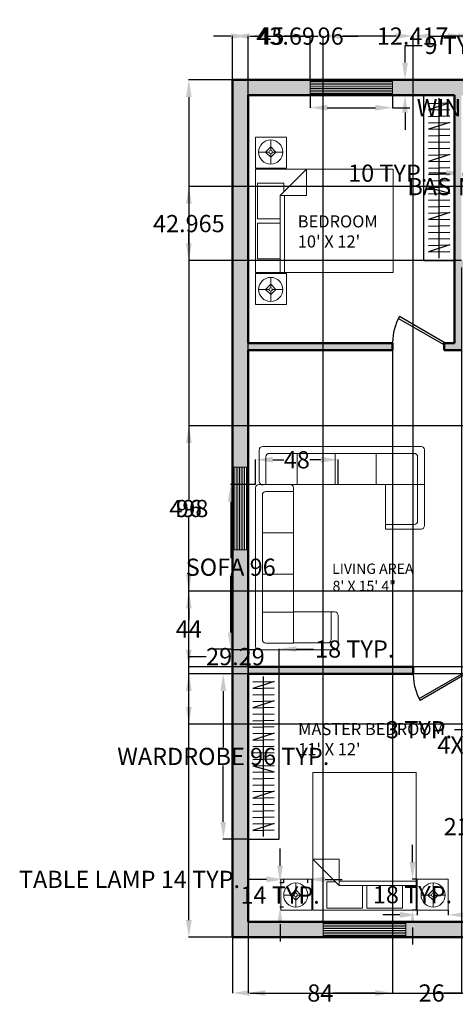
# Model space of a CAD drawing. Units: inches. Extents: x 133 to 758, y -29 to 543.
# Tile 1 of 7: x 133 to 386, y -29 to 543. Entities that reach past the tile are written whole.
import ezdxf

# ---------------------------------------------------------------- set-up
doc = ezdxf.new("R2010")
doc.units = ezdxf.units.IN
doc.header["$MEASUREMENT"] = 0
for name, color, linetype, lineweight in [('A-ANNO-DIMS', 2, 'Continuous', 18), ('A-AREA-IDEN', 7, 'Continuous', 25), ('A-FLOR-CASE', 32, 'Continuous', 25), ('A-FURN', 8, 'Continuous', 18), ('A-WALL', 7, 'Continuous', 50), ('DOOR', 40, 'Continuous', 25), ('WINDOW', 151, 'Continuous', 18)]:
    doc.layers.add(name, color=color, linetype=linetype, lineweight=lineweight)
doc.layers.add('A-WALL-PATT', color=251, linetype='Continuous', lineweight=13, true_color=0x636466)
doc.styles.get("Standard").update_dxf_attribs({"font": 'arial.ttf'})
doc.dimstyles.get("Standard").update_dxf_attribs({"dimtxt": 10, "dimasz": 10, "dimexe": 0.18, "dimexo": 0.0625, "dimgap": 0.09, "dimtad": 0, "dimtih": 1, "dimtoh": 1, "dimdec": 0, "dimzin": 0, "dimdsep": 46, "dimlunit": 4, "dimtxsty": 'Standard', "dimcen": 0.09, "dimadec": 0, "dimazin": 0, "dimtfac": 1, "dimtdec": 0, "dimtofl": 0, "dimtmove": 0, "dimatfit": 3, "dimfxl": 1, "dimtolj": 1, "dimtzin": 0, "dimarcsym": 0})

# ---------------------------------------------------------------- blocks, each defined once
blk = doc.blocks.new('*U14')
for p, q in [((0, 0), (0, -6)), ((-40, 0), (-40, -6))]:
    blk.add_line(p, q)
blk.add_lwpolyline([(0, 0), (-34.64, 20), (-35.52, 18.48), (-0.88, -1.52)], close=True)
blk.add_arc((0, 0), 40, 150, 180)
blk = doc.blocks.new('*U12')
for p, q in [((-40, 0), (-40, 6)), ((0, 0), (0, 6))]:
    blk.add_line(p, q)
blk.add_lwpolyline([(0, 0), (-34.64, -20), (-35.52, -18.48), (-0.88, 1.52)], close=True)
blk.add_arc((0, 0), 40, 180, 210)
blk = doc.blocks.new('SOFA')
for p, q in [((-1, 0), (1, 0)), ((1, 0), (17, 0)), ((-3, -2), (-3, -94)), ((19, -4), (3, -4)), ((19, -2), (19, -4)), ((43, -74), (41, -74)), ((41, -74), (41, -90)), ((45, -92), (45, -76)), ((-1, -96), (43, -96)), ((45, -92), (45, -94))]:
    blk.add_line(p, q)
blk.add_lwpolyline([(3, -4), (19.13, -4), (19.13, -28), (1, -28), (1, -6, -0.414214)], format="xyb", close=True)
for points in [[(39, -92), (19.13, -92), (19.13, -92.1), (3, -92.1, -0.414214), (1, -90.1), (1, -6)], [(1, -74.06), (19.13, -74.06), (19.13, -92), (39, -92, 0.414214), (41, -90), (41, -74), (19.13, -74), (19.13, -52), (1, -52), (1, -76)]]:
    blk.add_lwpolyline(points, format="xyb")
blk.add_lwpolyline([(1, -28), (19.13, -28), (19.13, -52), (1, -52)], close=True)
for centre, start, end in [((-1, -2), 90, 180), ((17, -2), 0, 90), ((43, -76), 0, 90), ((-1, -94), 180, 270), ((43, -94), 270, 0)]:
    blk.add_arc(centre, 2, start, end)
blk = doc.blocks.new('Bed - Queen')
for p, q in [((0, -80.00003), (0, 0)), ((0, 0), (59.99999, 0)), ((59.99999, 0), (59.99999, -80.00003)), ((7.99999, -1.2), (28.79998, -1.2)), ((7.99999, -14.4), (7.99999, -1.2)), ((28.79998, -1.2), (28.79998, -14.4)), ((31.19999, -1.2), (51.99999, -1.2)), ((31.19999, -14.4), (31.19999, -1.2)), ((51.99999, -1.2), (51.99999, -16.4)), ((0, -14.4), (44.8, -14.4)), ((44.8, -16.8), (0, -16.8)), ((59.99999, -29.6), (44.8, -14.4)), ((44.8, -14.4), (44.8, -29.6)), ((51.99999, -16.4), (46.79936, -16.4)), ((44.8, -29.6), (59.99999, -29.6)), ((59.99999, -80.00003), (0, -80.00003))]:
    blk.add_line(p, q)
blk = doc.blocks.new('Lamp - Table')
for p, q in [((0, 7), (0, 1)), ((-1, 0), (-7, 0)), ((0, 3), (-3, 0)), ((-3, 0), (0, -3)), ((3, 0), (0, 3)), ((0, -3), (3, 0)), ((1, 0), (7, 0)), ((0, -1), (0, -7))]:
    blk.add_line(p, q)
for radius in [7, 1]:
    blk.add_circle((0, 0), radius)
blk = doc.blocks.new('WIN-48IN')
for p, q in [((0, 8), (48, 8)), ((0, 7), (48, 7)), ((0, 6), (48, 6)), ((0, 5), (48, 5)), ((0, 4), (48, 4)), ((0, 3), (48, 3)), ((0, 2), (48, 2)), ((0, 1), (48, 1)), ((0, 0), (48, 0))]:
    blk.add_line(p, q)
blk.add_lwpolyline([(48, 9), (48, 0), (0, 0), (0, 9)], close=True)
blk = doc.blocks.new('WARDROBE-96X18IN')
for p, q in [((18, 96), (0, 96)), ((0, 96), (0, 0)), ((2.8, 91.24), (15.16, 91.53)), ((15.16, 91.53), (2.8, 87.49)), ((9, 1.47), (9, 94.4)), ((18, 0), (18, 96)), ((2.8, 87.49), (15.16, 87.78)), ((2.8, 83.75), (15.16, 84.04)), ((2.8, 80), (15.16, 80.29)), ((15.16, 80.29), (2.8, 76.25)), ((2.8, 76.25), (15.16, 76.54)), ((2.8, 72.51), (15.16, 72.8)), ((2.8, 68.76), (15.16, 69.05)), ((2.8, 65.01), (15.16, 65.3)), ((2.8, 61.27), (15.16, 61.56)), ((15.16, 61.56), (2.8, 57.52)), ((2.8, 57.52), (15.16, 57.81)), ((2.8, 53.77), (15.16, 54.06)), ((2.8, 50.03), (15.16, 50.32)), ((2.8, 46.28), (15.16, 46.57)), ((2.8, 42.53), (15.16, 42.82)), ((2.8, 42.53), (15.16, 39.08)), ((2.8, 38.79), (15.16, 39.08)), ((2.8, 35.04), (15.16, 35.33)), ((2.8, 31.29), (15.16, 31.58)), ((2.8, 27.55), (15.16, 27.84)), ((15.16, 27.84), (2.8, 23.8)), ((2.8, 23.8), (15.16, 24.09)), ((2.8, 20.06), (15.16, 20.35)), ((2.8, 16.31), (15.16, 16.6)), ((2.8, 12.56), (15.16, 12.85)), ((2.8, 8.82), (15.16, 9.11)), ((15.16, 9.11), (2.8, 5.07)), ((0, 0), (18, 0)), ((2.8, 5.07), (15.16, 5.36))]:
    blk.add_line(p, q)
blk = doc.blocks.new('NIGHTSTAND-18IN')
blk.add_lwpolyline([(18, 18), (18, 0), (0, 0), (0, 18)], close=True)
blk = doc.blocks.new('*D38')
at = {"layer": 'A-ANNO-DIMS', "color": 0, "lineweight": -2, "transparency": 16777216}
for p, q in [((276.46, 43.94), (266.46, 43.94)), ((286.46, 41.9), (286.46, 44.12)), ((300.46, 41.9), (300.46, 44.12)), ((310.46, 43.94), (320.46, 43.94))]:
    blk.add_line(p, q, dxfattribs=at)
at = {"layer": 'A-ANNO-DIMS', "color": 0, "transparency": 16777216}
for points in [[(276.46, 45.6), (276.46, 42.27), (286.46, 43.94)], [(310.46, 45.6), (310.46, 42.27), (300.46, 43.94)]]:
    blk.add_solid(points, dxfattribs=at)
at = {"layer": 'Defpoints', "color": 0, "transparency": 16777216}
for p in [(286.46, 43.94), (286.46, 41.84), (300.46, 41.84)]:
    blk.add_point(p, dxfattribs=at)
at = {"layer": 'A-ANNO-DIMS', "color": 0, "transparency": 16777216, "insert": (196.87, 43.94), "char_height": 10, "attachment_point": 5}
blk.add_mtext('\\A1;TABLE LAMP 14 TYP.', dxfattribs=at)
blk = doc.blocks.new('*D39')
at = {"layer": 'A-ANNO-DIMS', "color": 0, "lineweight": -2, "transparency": 16777216}
for p, q in [((284.36, 51.84), (284.36, 61.84)), ((286.4, 41.84), (284.18, 41.84)), ((286.4, 27.84), (284.18, 27.84)), ((284.36, 17.84), (284.36, 7.84))]:
    blk.add_line(p, q, dxfattribs=at)
at = {"layer": 'A-ANNO-DIMS', "color": 0, "transparency": 16777216}
for points in [[(282.69, 51.84), (286.02, 51.84), (284.36, 41.84)], [(282.69, 17.84), (286.02, 17.84), (284.36, 27.84)]]:
    blk.add_solid(points, dxfattribs=at)
at = {"layer": 'Defpoints', "color": 0, "transparency": 16777216}
for p in [(286.46, 41.84), (284.36, 27.84), (286.46, 27.84)]:
    blk.add_point(p, dxfattribs=at)
at = {"layer": 'A-ANNO-DIMS', "color": 0, "transparency": 16777216, "insert": (284.36, 34.84), "char_height": 10, "attachment_point": 5}
blk.add_mtext('\\A1;14 TYP.', dxfattribs=at)
blk = doc.blocks.new('*D40')
at = {"layer": 'A-ANNO-DIMS', "color": 0, "lineweight": -2, "transparency": 16777216}
for p, q in [((353.97, 23.32), (343.97, 23.32)), ((363.97, 25.96), (363.97, 23.14)), ((381.97, 25.96), (381.97, 23.14)), ((391.97, 23.32), (401.97, 23.32))]:
    blk.add_line(p, q, dxfattribs=at)
at = {"layer": 'A-ANNO-DIMS', "color": 0, "transparency": 16777216}
for points in [[(353.97, 24.99), (353.97, 21.65), (363.97, 23.32)], [(391.97, 24.99), (391.97, 21.65), (381.97, 23.32)]]:
    blk.add_solid(points, dxfattribs=at)
at = {"layer": 'Defpoints', "color": 0, "transparency": 16777216}
for p in [(363.97, 26.02), (381.97, 26.02), (381.97, 23.32)]:
    blk.add_point(p, dxfattribs=at)
at = {"layer": 'A-ANNO-DIMS', "color": 0, "transparency": 16777216, "insert": (473.5, 23.32), "char_height": 10, "attachment_point": 5}
blk.add_mtext('\\A1;NIGHTSTAND 18 TYP.', dxfattribs=at)
blk = doc.blocks.new('*D41')
at = {"layer": 'A-ANNO-DIMS', "color": 0, "lineweight": -2, "transparency": 16777216}
for p, q in [((361.27, 54.02), (361.27, 64.02)), ((363.9, 44.02), (361.09, 44.02)), ((363.9, 26.02), (361.09, 26.02)), ((361.27, 16.02), (361.27, 6.02))]:
    blk.add_line(p, q, dxfattribs=at)
at = {"layer": 'A-ANNO-DIMS', "color": 0, "transparency": 16777216}
for points in [[(359.6, 54.02), (362.93, 54.02), (361.27, 44.02)], [(359.6, 16.02), (362.93, 16.02), (361.27, 26.02)]]:
    blk.add_solid(points, dxfattribs=at)
at = {"layer": 'Defpoints', "color": 0, "transparency": 16777216}
for p in [(363.97, 44.02), (361.27, 26.02), (363.97, 26.02)]:
    blk.add_point(p, dxfattribs=at)
at = {"layer": 'A-ANNO-DIMS', "color": 0, "transparency": 16777216, "insert": (361.27, 35.02), "char_height": 10, "attachment_point": 5}
blk.add_mtext('\\A1;18 TYP.', dxfattribs=at)
blk = doc.blocks.new('*D42')
at = {"layer": 'A-ANNO-DIMS', "color": 0, "lineweight": -2, "transparency": 16777216}
for p, q in [((301.75, 499.27), (301.75, 491.96)), ((349.75, 499.27), (349.75, 491.96)), ((311.75, 492.14), (339.75, 492.14)), ((349.75, 492.14), (359.75, 492.14))]:
    blk.add_line(p, q, dxfattribs=at)
at = {"layer": 'A-ANNO-DIMS', "color": 0, "transparency": 16777216}
for points in [[(311.75, 493.8), (311.75, 490.47), (301.75, 492.14)], [(339.75, 493.8), (339.75, 490.47), (349.75, 492.14)]]:
    blk.add_solid(points, dxfattribs=at)
at = {"layer": 'Defpoints', "color": 0, "transparency": 16777216}
for p in [(301.75, 499.34), (349.75, 499.34), (349.75, 492.14)]:
    blk.add_point(p, dxfattribs=at)
at = {"layer": 'A-ANNO-DIMS', "color": 0, "transparency": 16777216, "insert": (416.97, 492.14), "char_height": 10, "attachment_point": 5}
blk.add_mtext('\\A1;WINDOW 48 TYP.', dxfattribs=at)
blk = doc.blocks.new('*D43')
at = {"layer": 'A-ANNO-DIMS', "color": 0, "lineweight": -2, "transparency": 16777216}
for p, q in [((356.95, 518.34), (356.95, 528.34)), ((356.95, 528.34), (366.95, 528.34)), ((349.81, 508.34), (357.13, 508.34)), ((349.81, 499.34), (357.13, 499.34)), ((356.95, 489.34), (356.95, 479.34))]:
    blk.add_line(p, q, dxfattribs=at)
at = {"layer": 'A-ANNO-DIMS', "color": 0, "transparency": 16777216}
for points in [[(355.28, 518.34), (358.62, 518.34), (356.95, 508.34)], [(355.28, 489.34), (358.62, 489.34), (356.95, 499.34)]]:
    blk.add_solid(points, dxfattribs=at)
at = {"layer": 'Defpoints', "color": 0, "transparency": 16777216}
for p in [(349.75, 508.34), (356.95, 508.34), (349.75, 499.34)]:
    blk.add_point(p, dxfattribs=at)
at = {"layer": 'A-ANNO-DIMS', "color": 0, "transparency": 16777216, "insert": (387.49, 528.34), "char_height": 10, "attachment_point": 5}
blk.add_mtext('\\A1;9 TYP.', dxfattribs=at)
blk = doc.blocks.new('*D46')
at = {"layer": 'A-ANNO-DIMS', "color": 0, "lineweight": -2, "transparency": 16777216}
for p, q in [((265.69, 163.34), (251.17, 163.34)), ((251.35, 153.34), (251.35, 120.6)), ((251.35, 77.34), (251.35, 110.07)), ((265.69, 67.34), (251.17, 67.34))]:
    blk.add_line(p, q, dxfattribs=at)
at = {"layer": 'A-ANNO-DIMS', "color": 0, "transparency": 16777216}
for points in [[(249.68, 153.34), (253.02, 153.34), (251.35, 163.34)], [(249.68, 77.34), (253.02, 77.34), (251.35, 67.34)]]:
    blk.add_solid(points, dxfattribs=at)
at = {"layer": 'Defpoints', "color": 0, "transparency": 16777216}
for p in [(251.35, 163.34), (265.75, 163.34), (265.75, 67.34)]:
    blk.add_point(p, dxfattribs=at)
at = {"layer": 'A-ANNO-DIMS', "color": 0, "transparency": 16777216, "insert": (251.35, 115.34), "char_height": 10, "attachment_point": 5}
blk.add_mtext('\\A1;WARDROBE 96 TYP.', dxfattribs=at)
blk = doc.blocks.new('*D47')
at = {"layer": 'A-ANNO-DIMS', "color": 0, "lineweight": -2, "transparency": 16777216}
for p, q in [((255.75, 177.74), (245.75, 177.74)), ((265.75, 163.4), (265.75, 177.92)), ((283.75, 163.4), (283.75, 177.92)), ((293.75, 177.74), (303.75, 177.74))]:
    blk.add_line(p, q, dxfattribs=at)
at = {"layer": 'A-ANNO-DIMS', "color": 0, "transparency": 16777216}
for points in [[(255.75, 179.4), (255.75, 176.07), (265.75, 177.74)], [(293.75, 179.4), (293.75, 176.07), (283.75, 177.74)]]:
    blk.add_solid(points, dxfattribs=at)
at = {"layer": 'Defpoints', "color": 0, "transparency": 16777216}
for p in [(283.75, 177.74), (265.75, 163.34), (283.75, 163.34)]:
    blk.add_point(p, dxfattribs=at)
at = {"layer": 'A-ANNO-DIMS', "color": 0, "transparency": 16777216, "insert": (327.71, 177.74), "char_height": 10, "attachment_point": 5}
blk.add_mtext('\\A1;18 TYP.', dxfattribs=at)
blk = doc.blocks.new('*D51')
at = {"layer": 'A-ANNO-DIMS', "color": 0, "lineweight": -2, "transparency": 16777216}
for p, q in [((441.86, 105.57), (436.79, 105.57)), ((436.97, 95.57), (436.97, 94.57)), ((441.86, 84.57), (436.79, 84.57)), ((436.97, 84.57), (436.97, 74.57)), ((436.97, 74.57), (426.97, 74.57))]:
    blk.add_line(p, q, dxfattribs=at)
at = {"layer": 'A-ANNO-DIMS', "color": 0, "transparency": 16777216}
for points in [[(435.3, 95.57), (438.63, 95.57), (436.97, 105.57)], [(435.3, 94.57), (438.63, 94.57), (436.97, 84.57)]]:
    blk.add_solid(points, dxfattribs=at)
at = {"layer": 'Defpoints', "color": 0, "transparency": 16777216}
for p in [(441.92, 105.57), (436.97, 84.57), (441.92, 84.57)]:
    blk.add_point(p, dxfattribs=at)
at = {"layer": 'A-ANNO-DIMS', "color": 0, "transparency": 16777216, "insert": (402.45, 74.57), "char_height": 10, "attachment_point": 5}
blk.add_mtext('\\A1;21 TYP.', dxfattribs=at)
blk = doc.blocks.new('*D52')
at = {"layer": 'A-ANNO-DIMS', "color": 0, "lineweight": -2, "transparency": 16777216}
for p, q in [((402.53, 462.32), (402.53, 472.32)), ((400.79, 452.32), (402.71, 452.32)), ((400.79, 440.28), (402.71, 440.28)), ((402.53, 430.28), (402.53, 420.28))]:
    blk.add_line(p, q, dxfattribs=at)
at = {"layer": 'A-ANNO-DIMS', "color": 0, "transparency": 16777216}
for points in [[(400.87, 462.32), (404.2, 462.32), (402.53, 452.32)], [(400.87, 430.28), (404.2, 430.28), (402.53, 440.28)]]:
    blk.add_solid(points, dxfattribs=at)
at = {"layer": 'Defpoints', "color": 0, "transparency": 16777216}
for p in [(400.73, 452.32), (402.53, 452.32), (400.73, 440.28)]:
    blk.add_point(p, dxfattribs=at)
at = {"layer": 'A-ANNO-DIMS', "color": 0, "transparency": 16777216, "insert": (402.53, 446.3), "char_height": 10, "attachment_point": 5}
blk.add_mtext('\\A1;BASIN 12 TYP.', dxfattribs=at)
blk = doc.blocks.new('*D53')
at = {"layer": 'A-ANNO-DIMS', "color": 0, "lineweight": -2, "transparency": 16777216}
for p, q in [((380.86, 454.12), (370.86, 454.12)), ((390.86, 452.38), (390.86, 454.3)), ((400.73, 452.38), (400.73, 454.3)), ((410.73, 454.12), (420.73, 454.12))]:
    blk.add_line(p, q, dxfattribs=at)
at = {"layer": 'A-ANNO-DIMS', "color": 0, "transparency": 16777216}
for points in [[(380.86, 455.79), (380.86, 452.46), (390.86, 454.12)], [(410.73, 455.79), (410.73, 452.46), (400.73, 454.12)]]:
    blk.add_solid(points, dxfattribs=at)
at = {"layer": 'Defpoints', "color": 0, "transparency": 16777216}
for p in [(390.86, 454.12), (390.86, 452.32), (400.73, 452.32)]:
    blk.add_point(p, dxfattribs=at)
at = {"layer": 'A-ANNO-DIMS', "color": 0, "transparency": 16777216, "insert": (346.9, 454.12), "char_height": 10, "attachment_point": 5}
blk.add_mtext('\\A1;10 TYP.', dxfattribs=at)
blk = doc.blocks.new('*D55')
at = {"layer": 'A-ANNO-DIMS', "color": 0, "lineweight": -2, "transparency": 16777216}
for p, q in [((405.63, 131.53), (405.63, 130.68)), ((408.82, 131.53), (408.82, 130.68)), ((395.63, 130.86), (385.63, 130.86)), ((418.82, 130.86), (428.82, 130.86))]:
    blk.add_line(p, q, dxfattribs=at)
at = {"layer": 'A-ANNO-DIMS', "color": 0, "transparency": 16777216}
for points in [[(395.63, 132.53), (395.63, 129.19), (405.63, 130.86)], [(418.82, 132.53), (418.82, 129.19), (408.82, 130.86)]]:
    blk.add_solid(points, dxfattribs=at)
at = {"layer": 'Defpoints', "color": 0, "transparency": 16777216}
for p in [(405.63, 131.6), (408.82, 131.6), (405.63, 130.86)]:
    blk.add_point(p, dxfattribs=at)
at = {"layer": 'A-ANNO-DIMS', "color": 0, "transparency": 16777216, "insert": (365.09, 130.86), "char_height": 10, "attachment_point": 5}
blk.add_mtext('\\A1;3 TYP.', dxfattribs=at)
blk = doc.blocks.new('*D70')
at = {"layer": 'A-ANNO-DIMS', "color": 0, "lineweight": -2, "transparency": 16777216}
for p, q in [((270.02, 273.25), (255.5, 273.25)), ((255.68, 263.25), (255.68, 230.52)), ((255.68, 187.25), (255.68, 219.99)), ((270.02, 177.25), (255.5, 177.25))]:
    blk.add_line(p, q, dxfattribs=at)
at = {"layer": 'A-ANNO-DIMS', "color": 0, "transparency": 16777216}
for points in [[(254.02, 263.25), (257.35, 263.25), (255.68, 273.25)], [(254.02, 187.25), (257.35, 187.25), (255.68, 177.25)]]:
    blk.add_solid(points, dxfattribs=at)
at = {"layer": 'Defpoints', "color": 0, "transparency": 16777216}
for p in [(255.68, 273.25), (270.08, 273.25), (270.08, 177.25)]:
    blk.add_point(p, dxfattribs=at)
at = {"layer": 'A-ANNO-DIMS', "color": 0, "transparency": 16777216, "insert": (255.68, 225.25), "char_height": 10, "attachment_point": 5}
blk.add_mtext('\\A1;SOFA 96', dxfattribs=at)
blk = doc.blocks.new('*D71')
at = {"layer": 'A-ANNO-DIMS', "color": 0, "lineweight": -2, "transparency": 16777216}
for p, q in [((270.08, 273.31), (270.08, 287.83)), ((280.08, 287.65), (286.62, 287.65)), ((308.08, 287.65), (301.55, 287.65)), ((318.08, 273.31), (318.08, 287.83))]:
    blk.add_line(p, q, dxfattribs=at)
at = {"layer": 'A-ANNO-DIMS', "color": 0, "transparency": 16777216}
for points in [[(280.08, 289.32), (280.08, 285.99), (270.08, 287.65)], [(308.08, 289.32), (308.08, 285.99), (318.08, 287.65)]]:
    blk.add_solid(points, dxfattribs=at)
at = {"layer": 'Defpoints', "color": 0, "transparency": 16777216}
for p in [(318.08, 287.65), (270.08, 273.25), (318.08, 273.25)]:
    blk.add_point(p, dxfattribs=at)
at = {"layer": 'A-ANNO-DIMS', "color": 0, "transparency": 16777216, "insert": (294.08, 287.65), "char_height": 10, "attachment_point": 5}
blk.add_mtext('\\A1;48', dxfattribs=at)
blk = doc.blocks.new('*D72')
at = {"layer": 'A-ANNO-DIMS', "color": 0, "lineweight": -2, "transparency": 16777216}
for p, q in [((256.75, 10.27), (256.75, -22.24)), ((634.75, 10.27), (634.75, -22.24)), ((266.75, -22.06), (434.61, -22.06)), ((624.75, -22.06), (456.89, -22.06))]:
    blk.add_line(p, q, dxfattribs=at)
at = {"layer": 'A-ANNO-DIMS', "color": 0, "transparency": 16777216}
for points in [[(266.75, -20.4), (266.75, -23.73), (256.75, -22.06)], [(624.75, -20.4), (624.75, -23.73), (634.75, -22.06)]]:
    blk.add_solid(points, dxfattribs=at)
at = {"layer": 'Defpoints', "color": 0, "transparency": 16777216}
for p in [(256.75, 10.34), (634.75, 10.34), (634.75, -22.06)]:
    blk.add_point(p, dxfattribs=at)
at = {"layer": 'A-ANNO-DIMS', "color": 0, "transparency": 16777216, "insert": (445.75, -22.06), "char_height": 10, "attachment_point": 5}
blk.add_mtext('\\A1;378', dxfattribs=at)
blk = doc.blocks.new('*D73')
at = {"layer": 'A-ANNO-DIMS', "color": 0, "lineweight": -2, "transparency": 16777216}
for p, q in [((256.69, 508.34), (231.17, 508.34)), ((231.35, 498.34), (231.35, 264.53)), ((231.35, 20.34), (231.35, 254.14)), ((256.69, 10.34), (231.17, 10.34))]:
    blk.add_line(p, q, dxfattribs=at)
at = {"layer": 'A-ANNO-DIMS', "color": 0, "transparency": 16777216}
for points in [[(229.68, 498.34), (233.02, 498.34), (231.35, 508.34)], [(229.68, 20.34), (233.02, 20.34), (231.35, 10.34)]]:
    blk.add_solid(points, dxfattribs=at)
at = {"layer": 'Defpoints', "color": 0, "transparency": 16777216}
for p in [(231.35, 508.34), (256.75, 508.34), (256.75, 10.34)]:
    blk.add_point(p, dxfattribs=at)
at = {"layer": 'A-ANNO-DIMS', "color": 0, "transparency": 16777216, "insert": (231.35, 259.34), "char_height": 10, "attachment_point": 5}
blk.add_mtext('\\A1;498', dxfattribs=at)
blk = doc.blocks.new('*D75')
at = {"layer": 'A-ANNO-DIMS', "color": 0, "lineweight": -2, "transparency": 16777216}
for p, q in [((525.69, 307.34), (231.17, 307.34)), ((231.35, 297.34), (231.35, 264.53)), ((231.35, 221.34), (231.35, 254.14)), ((525.69, 211.34), (231.17, 211.34))]:
    blk.add_line(p, q, dxfattribs=at)
at = {"layer": 'A-ANNO-DIMS', "color": 0, "transparency": 16777216}
for points in [[(229.68, 297.34), (233.02, 297.34), (231.35, 307.34)], [(229.68, 221.34), (233.02, 221.34), (231.35, 211.34)]]:
    blk.add_solid(points, dxfattribs=at)
at = {"layer": 'Defpoints', "color": 0, "transparency": 16777216}
for p in [(231.35, 307.34), (525.75, 307.34), (525.75, 211.34)]:
    blk.add_point(p, dxfattribs=at)
at = {"layer": 'A-ANNO-DIMS', "color": 0, "transparency": 16777216, "insert": (231.35, 259.34), "char_height": 10, "attachment_point": 5}
blk.add_mtext('\\A1;96', dxfattribs=at)
blk = doc.blocks.new('*D76')
at = {"layer": 'A-ANNO-DIMS', "color": 0, "lineweight": -2, "transparency": 16777216}
for p, q in [((525.69, 211.34), (231.17, 211.34)), ((231.35, 201.34), (231.35, 194.43)), ((231.35, 177.34), (231.35, 184.25)), ((525.69, 167.34), (231.17, 167.34))]:
    blk.add_line(p, q, dxfattribs=at)
at = {"layer": 'A-ANNO-DIMS', "color": 0, "transparency": 16777216}
for points in [[(229.68, 201.34), (233.02, 201.34), (231.35, 211.34)], [(229.68, 177.34), (233.02, 177.34), (231.35, 167.34)]]:
    blk.add_solid(points, dxfattribs=at)
at = {"layer": 'Defpoints', "color": 0, "transparency": 16777216}
for p in [(231.35, 211.34), (525.75, 211.34), (525.75, 167.34)]:
    blk.add_point(p, dxfattribs=at)
at = {"layer": 'A-ANNO-DIMS', "color": 0, "transparency": 16777216, "insert": (231.35, 189.34), "char_height": 10, "attachment_point": 5}
blk.add_mtext('\\A1;44', dxfattribs=at)
blk = doc.blocks.new('*D77')
at = {"layer": 'A-ANNO-DIMS', "color": 0, "lineweight": -2, "transparency": 16777216}
for p, q in [((265.75, 167.4), (265.75, 533.92)), ((275.75, 533.74), (306.5, 533.74)), ((351.75, 533.74), (321, 533.74)), ((361.75, 167.4), (361.75, 533.92))]:
    blk.add_line(p, q, dxfattribs=at)
at = {"layer": 'A-ANNO-DIMS', "color": 0, "transparency": 16777216}
for points in [[(275.75, 535.4), (275.75, 532.07), (265.75, 533.74)], [(351.75, 535.4), (351.75, 532.07), (361.75, 533.74)]]:
    blk.add_solid(points, dxfattribs=at)
at = {"layer": 'Defpoints', "color": 0, "transparency": 16777216}
for p in [(361.75, 533.74), (265.75, 167.34), (361.75, 167.34)]:
    blk.add_point(p, dxfattribs=at)
at = {"layer": 'A-ANNO-DIMS', "color": 0, "transparency": 16777216, "insert": (313.75, 533.74), "char_height": 10, "attachment_point": 5}
blk.add_mtext('\\A1;96', dxfattribs=at)
blk = doc.blocks.new('*D78')
at = {"layer": 'A-ANNO-DIMS', "color": 0, "lineweight": -2, "transparency": 16777216}
for p, q in [((361.75, 167.4), (361.75, 533.92)), ((371.75, 533.74), (381.75, 533.74)), ((391.75, 167.4), (391.75, 533.92)), ((391.75, 533.74), (401.75, 533.74))]:
    blk.add_line(p, q, dxfattribs=at)
at = {"layer": 'A-ANNO-DIMS', "color": 0, "transparency": 16777216}
for points in [[(371.75, 535.4), (371.75, 532.07), (361.75, 533.74)], [(381.75, 535.4), (381.75, 532.07), (391.75, 533.74)]]:
    blk.add_solid(points, dxfattribs=at)
at = {"layer": 'Defpoints', "color": 0, "transparency": 16777216}
for p in [(391.75, 533.74), (361.75, 167.34), (391.75, 167.34)]:
    blk.add_point(p, dxfattribs=at)
at = {"layer": 'A-ANNO-DIMS', "color": 0, "transparency": 16777216, "insert": (408.98, 533.74), "char_height": 10, "attachment_point": 5}
blk.add_mtext('\\A1;30', dxfattribs=at)
blk = doc.blocks.new('*D79')
at = {"layer": 'A-ANNO-DIMS', "color": 0, "lineweight": -2, "transparency": 16777216}
for p, q in [((256.75, 508.4), (256.75, 533.92)), ((266.75, 533.74), (271.76, 533.74)), ((291.75, 533.74), (286.74, 533.74)), ((301.75, 508.4), (301.75, 533.92))]:
    blk.add_line(p, q, dxfattribs=at)
at = {"layer": 'A-ANNO-DIMS', "color": 0, "transparency": 16777216}
for points in [[(266.75, 535.4), (266.75, 532.07), (256.75, 533.74)], [(291.75, 535.4), (291.75, 532.07), (301.75, 533.74)]]:
    blk.add_solid(points, dxfattribs=at)
at = {"layer": 'Defpoints', "color": 0, "transparency": 16777216}
for p in [(301.75, 533.74), (256.75, 508.34), (301.75, 508.34)]:
    blk.add_point(p, dxfattribs=at)
at = {"layer": 'A-ANNO-DIMS', "color": 0, "transparency": 16777216, "insert": (279.25, 533.74), "char_height": 10, "attachment_point": 5}
blk.add_mtext('\\A1;45', dxfattribs=at)
blk = doc.blocks.new('*D83')
at = {"layer": 'A-ANNO-DIMS', "color": 0, "lineweight": -2, "transparency": 16777216}
for p, q in [((255.75, 533.74), (245.75, 533.74)), ((265.75, 19.4), (265.75, 533.92)), ((309.44, 19.4), (309.44, 533.92)), ((319.44, 533.74), (329.44, 533.74))]:
    blk.add_line(p, q, dxfattribs=at)
at = {"layer": 'A-ANNO-DIMS', "color": 0, "transparency": 16777216}
for points in [[(255.75, 535.4), (255.75, 532.07), (265.75, 533.74)], [(319.44, 535.4), (319.44, 532.07), (309.44, 533.74)]]:
    blk.add_solid(points, dxfattribs=at)
at = {"layer": 'Defpoints', "color": 0, "transparency": 16777216}
for p in [(309.44, 533.74), (265.75, 19.34), (309.44, 19.34)]:
    blk.add_point(p, dxfattribs=at)
at = {"layer": 'A-ANNO-DIMS', "color": 0, "transparency": 16777216, "insert": (287.59, 533.74), "char_height": 10, "attachment_point": 5}
blk.add_mtext('\\A1;43.69', dxfattribs=at)
blk = doc.blocks.new('*D85')
at = {"layer": 'A-ANNO-DIMS', "color": 0, "lineweight": -2, "transparency": 16777216}
for p, q in [((389.75, 399.27), (389.75, -22.24)), ((415.75, 399.27), (415.75, -22.24)), ((389.75, -22.06), (379.75, -22.06)), ((405.75, -22.06), (399.75, -22.06))]:
    blk.add_line(p, q, dxfattribs=at)
at = {"layer": 'A-ANNO-DIMS', "color": 0, "transparency": 16777216}
for points in [[(399.75, -20.4), (399.75, -23.73), (389.75, -22.06)], [(405.75, -20.4), (405.75, -23.73), (415.75, -22.06)]]:
    blk.add_solid(points, dxfattribs=at)
at = {"layer": 'Defpoints', "color": 0, "transparency": 16777216}
for p in [(389.75, 399.34), (415.75, 399.34), (389.75, -22.06)]:
    blk.add_point(p, dxfattribs=at)
at = {"layer": 'A-ANNO-DIMS', "color": 0, "transparency": 16777216, "insert": (372.42, -22.06), "char_height": 10, "attachment_point": 5}
blk.add_mtext('\\A1;26', dxfattribs=at)
blk = doc.blocks.new('*D87')
at = {"layer": 'A-ANNO-DIMS', "color": 0, "lineweight": -2, "transparency": 16777216}
for p, q in [((265.75, 351.27), (265.75, -22.24)), ((349.75, 351.27), (349.75, -22.24)), ((275.75, -22.06), (300.51, -22.06)), ((339.75, -22.06), (314.99, -22.06))]:
    blk.add_line(p, q, dxfattribs=at)
at = {"layer": 'A-ANNO-DIMS', "color": 0, "transparency": 16777216}
for points in [[(275.75, -20.4), (275.75, -23.73), (265.75, -22.06)], [(339.75, -20.4), (339.75, -23.73), (349.75, -22.06)]]:
    blk.add_solid(points, dxfattribs=at)
at = {"layer": 'Defpoints', "color": 0, "transparency": 16777216}
for p in [(265.75, 351.34), (349.75, 351.34), (349.75, -22.06)]:
    blk.add_point(p, dxfattribs=at)
at = {"layer": 'A-ANNO-DIMS', "color": 0, "transparency": 16777216, "insert": (307.75, -22.06), "char_height": 10, "attachment_point": 5}
blk.add_mtext('\\A1;84', dxfattribs=at)
blk = doc.blocks.new('*D89')
at = {"layer": 'A-ANNO-DIMS', "color": 0, "lineweight": -2, "transparency": 16777216}
for p, q in [((387.75, 533.74), (377.75, 533.74)), ((397.75, 163.4), (397.75, 533.92)), ((401.75, 163.4), (401.75, 533.92)), ((411.75, 533.74), (421.75, 533.74))]:
    blk.add_line(p, q, dxfattribs=at)
at = {"layer": 'A-ANNO-DIMS', "color": 0, "transparency": 16777216}
for points in [[(387.75, 535.4), (387.75, 532.07), (397.75, 533.74)], [(411.75, 535.4), (411.75, 532.07), (401.75, 533.74)]]:
    blk.add_solid(points, dxfattribs=at)
at = {"layer": 'Defpoints', "color": 0, "transparency": 16777216}
for p in [(401.75, 533.74), (397.75, 163.34), (401.75, 163.34)]:
    blk.add_point(p, dxfattribs=at)
at = {"layer": 'A-ANNO-DIMS', "color": 0, "transparency": 16777216, "insert": (425.3, 533.74), "char_height": 10, "attachment_point": 5}
blk.add_mtext('\\A1;4', dxfattribs=at)
blk = doc.blocks.new('*D92')
at = {"layer": 'A-ANNO-DIMS', "color": 0, "lineweight": -2, "transparency": 16777216}
for p, q in [((395.73, 446.3), (231.17, 446.3)), ((231.35, 436.3), (231.35, 430.01)), ((231.35, 413.34), (231.35, 419.62)), ((389.69, 403.34), (231.17, 403.34))]:
    blk.add_line(p, q, dxfattribs=at)
at = {"layer": 'A-ANNO-DIMS', "color": 0, "transparency": 16777216}
for points in [[(229.68, 436.3), (233.02, 436.3), (231.35, 446.3)], [(229.68, 413.34), (233.02, 413.34), (231.35, 403.34)]]:
    blk.add_solid(points, dxfattribs=at)
at = {"layer": 'Defpoints', "color": 0, "transparency": 16777216}
for p in [(395.79, 446.3), (231.35, 403.34), (389.75, 403.34)]:
    blk.add_point(p, dxfattribs=at)
at = {"layer": 'A-ANNO-DIMS', "color": 0, "transparency": 16777216, "insert": (231.35, 424.82), "char_height": 10, "attachment_point": 5}
blk.add_mtext('\\A1;42.965', dxfattribs=at)
blk = doc.blocks.new('*D96')
at = {"layer": 'A-ANNO-DIMS', "color": 0, "lineweight": -2, "transparency": 16777216}
for p, q in [((231.35, 163.34), (231.35, 173.34)), ((231.35, 173.34), (241.35, 173.34)), ((401.69, 163.34), (231.17, 163.34)), ((231.35, 144.05), (231.35, 153.34)), ((408.73, 134.05), (231.17, 134.05))]:
    blk.add_line(p, q, dxfattribs=at)
at = {"layer": 'A-ANNO-DIMS', "color": 0, "transparency": 16777216}
for points in [[(229.68, 153.34), (233.02, 153.34), (231.35, 163.34)], [(229.68, 144.05), (233.02, 144.05), (231.35, 134.05)]]:
    blk.add_solid(points, dxfattribs=at)
at = {"layer": 'Defpoints', "color": 0, "transparency": 16777216}
for p in [(231.35, 163.34), (401.75, 163.34), (408.8, 134.05)]:
    blk.add_point(p, dxfattribs=at)
at = {"layer": 'A-ANNO-DIMS', "color": 0, "transparency": 16777216, "insert": (258.41, 173.34), "char_height": 10, "attachment_point": 5}
blk.add_mtext('\\A1;29.29', dxfattribs=at)
blk = doc.blocks.new('*D99')
at = {"layer": 'A-ANNO-DIMS', "color": 0, "lineweight": -2, "transparency": 16777216}
for p, q in [((391.75, 533.74), (381.75, 533.74)), ((401.75, 19.4), (401.75, 533.92)), ((414.17, 21.95), (414.17, 533.92)), ((424.17, 533.74), (434.17, 533.74))]:
    blk.add_line(p, q, dxfattribs=at)
at = {"layer": 'A-ANNO-DIMS', "color": 0, "transparency": 16777216}
for points in [[(391.75, 535.4), (391.75, 532.07), (401.75, 533.74)], [(424.17, 535.4), (424.17, 532.07), (414.17, 533.74)]]:
    blk.add_solid(points, dxfattribs=at)
at = {"layer": 'Defpoints', "color": 0, "transparency": 16777216}
for p in [(401.75, 533.74), (401.75, 19.34), (414.17, 21.89)]:
    blk.add_point(p, dxfattribs=at)
at = {"layer": 'A-ANNO-DIMS', "color": 0, "transparency": 16777216, "insert": (361.37, 533.74), "char_height": 10, "attachment_point": 5}
blk.add_mtext('\\A1;12.417', dxfattribs=at)
blk = doc.blocks.new('*D102')
at = {"layer": 'A-ANNO-DIMS', "color": 0, "lineweight": -2, "transparency": 16777216}
for p, q in [((438.98, 121.92), (448.98, 121.92)), ((448.98, 121.92), (450.31, 112.01)), ((453.06, 90.87), (453.24, 90.87)), ((453.15, 90.78), (453.15, 90.96))]:
    blk.add_line(p, q, dxfattribs=at)
at = {"layer": 'A-ANNO-DIMS', "color": 0, "transparency": 16777216}
blk.add_solid([(451.96, 112.23), (448.66, 111.79), (451.64, 102.1)], dxfattribs=at)
at = {"layer": 'Defpoints', "color": 0, "transparency": 16777216}
for p in [(451.64, 102.1), (453.15, 90.87)]:
    blk.add_point(p, dxfattribs=at)
at = {"layer": 'A-ANNO-DIMS', "color": 0, "transparency": 16777216, "insert": (406.29, 121.92), "char_height": 10, "attachment_point": 5}
blk.add_mtext('\\A1;4X R11.33', dxfattribs=at)

msp = doc.modelspace()

# ---------------------------------------------------------------- hatches: boundary and pattern name
at = {"layer": 'A-WALL-PATT'}
h = msp.add_hatch(color=256, dxfattribs=at)
h.dxf.hatch_style = 1
h.paths.add_polyline_path([(433.7501, 508.336), (349.7501, 508.336), (349.7501, 499.336), (385.7501, 499.336), (385.7501, 403.336), (385.7501, 355.336), (379.7501, 355.336), (379.7501, 351.336), (389.7501, 351.336), (389.7501, 399.336), (415.7501, 399.336), (415.7501, 403.336), (389.7501, 403.336), (389.7501, 499.336), (433.7501, 499.336)])
h.paths.add_polyline_path([(541.7501, 508.336), (457.7501, 508.336), (457.7501, 499.336), (491.7501, 499.336), (491.7501, 403.336), (445.7501, 403.336), (445.7501, 399.336), (491.7501, 399.336), (491.7501, 351.336), (495.7501, 351.336), (495.7501, 399.336), (495.7501, 499.336), (513.7501, 499.336), (541.7501, 499.336)])
h.paths.add_polyline_path([(634.7501, 508.336), (589.7501, 508.336), (589.7501, 499.336), (625.7501, 499.336), (625.7501, 355.336), (525.7501, 355.336), (525.7501, 351.336), (525.7501, 307.336), (529.7501, 307.336), (529.7501, 351.336), (625.7501, 351.336), (625.7501, 283.336), (634.7501, 283.336)])
h.paths.add_polyline_path([(301.7501, 508.336), (256.7501, 508.336), (256.7501, 283.336), (265.7501, 283.336), (265.7501, 351.336), (349.7501, 351.336), (349.7501, 355.336), (265.7501, 355.336), (265.7501, 499.336), (301.7501, 499.336)])
h.paths.add_polyline_path([(361.7501, 167.336), (265.7501, 167.336), (265.7501, 235.336), (256.7501, 235.336), (256.7501, 10.336), (309.4362, 10.336), (309.4362, 19.336), (265.7501, 19.336), (265.7501, 163.336), (283.7501, 163.336), (361.7501, 163.336)])
h = msp.add_hatch(color=256, dxfattribs=at)
h.dxf.hatch_style = 1
h.paths.add_polyline_path([(425.9734, 19.336), (401.7501, 19.336), (401.7501, 163.336), (403.7501, 163.336), (403.7501, 167.336), (391.7501, 167.336), (391.7501, 163.336), (397.7501, 163.336), (397.7501, 19.336), (357.4362, 19.336), (357.4362, 10.336), (425.9734, 10.336)])

# ---------------------------------------------------------------- linework, layer by layer
at = {"layer": 'A-FURN'}
for p, q in [((364.2714, 273.383), (364.2714, 289.383)), ((362.2714, 250.0245), (345.6968, 250.0245))]:
    msp.add_line(p, q, dxfattribs=at)
for points in [[(368.2714, 291.383), (368.2714, 293.383, 0.41421356), (366.2714, 295.383), (274.2714, 295.383, 0.41421356), (272.2714, 293.383), (272.2714, 275.0794, 0.44250054), (274.4623, 273.0886), (276.1671, 273.252)], [(294.2151, 291.383), (294.2151, 273.252), (276.2714, 273.252), (276.1671, 273.252), (276.1671, 289.383, -0.41421356), (278.1671, 291.383), (362.2714, 291.383)]]:
    msp.add_lwpolyline(points, format="xyb", dxfattribs=at)
for points in [[(294.2714, 273.252), (316.2714, 273.252), (316.2714, 291.383), (292.2714, 291.383)], [(368.2714, 271.252), (368.2714, 249.383), (368.2714, 291.383), (368.2714, 275.383)], [(366.2714, 247.383), (345.6968, 247.383), (345.6968, 273.252)], [(366.2714, 273.252), (364.2714, 273.252), (348.2714, 273.252)], [(368.2714, 273.252), (364.2714, 273.252), (364.2714, 252.0245)]]:
    msp.add_lwpolyline(points, dxfattribs=at)
msp.add_lwpolyline([(340.2714, 291.383), (340.2714, 273.252), (316.2714, 273.252), (316.2714, 291.383)], close=True, dxfattribs=at)
msp.add_lwpolyline([(364.2714, 289.383), (364.2714, 273.252), (340.2714, 273.252), (340.2714, 291.383), (362.2714, 291.383, -0.41421356)], format="xyb", close=True, dxfattribs=at)
for centre in [(362.2714, 252.0245), (366.2714, 249.383)]:
    msp.add_arc(centre, 2, 270, 0, dxfattribs=at)
at = {"layer": 'A-WALL'}
for p, q in [((265.7501, 499.336), (385.7501, 499.336)), ((265.7501, 355.336), (265.7501, 499.336)), ((385.7501, 355.336), (385.7501, 499.336)), ((265.7501, 355.336), (349.7501, 355.336)), ((349.7501, 355.336), (349.7501, 351.336)), ((379.7501, 355.336), (379.7501, 351.336)), ((379.7501, 355.336), (385.7501, 355.336)), ((265.7501, 351.336), (349.7501, 351.336)), ((265.7501, 167.336), (265.7501, 351.336)), ((379.7501, 351.336), (389.7501, 351.336)), ((361.7501, 167.336), (265.7501, 167.336)), ((361.7501, 163.336), (361.7501, 167.336)), ((265.7501, 19.336), (265.7501, 163.336)), ((361.7501, 163.336), (265.7501, 163.336)), ((397.7501, 19.336), (265.7501, 19.336))]:
    msp.add_line(p, q, dxfattribs=at)
msp.add_lwpolyline([(505.7501, 10.336), (256.7501, 10.336), (256.7501, 508.336), (634.7501, 508.336), (634.7501, 10.336), (601.3503, 10.336)], dxfattribs=at)

# ---------------------------------------------------------------- block references
at = {"layer": 'A-FLOR-CASE'}
for p in [(367.75, 403.336), (265.75, 67.336)]:
    msp.add_blockref('WARDROBE-96X18IN', p, dxfattribs=at)
at = {"layer": 'A-FURN'}
for name, p, rotation in [('NIGHTSTAND-18IN', (288.074, 474.9676), 180), ('Lamp - Table', (278.8918, 466.3768), 90), ('Bed - Queen', (270.0735, 396.36), 90), ('NIGHTSTAND-18IN', (288.074, 395.8678), 180), ('Lamp - Table', (278.9002, 386.5709), 90), ('Bed - Queen', (363.4748, 26.0197), 180), ('NIGHTSTAND-18IN', (284.8672, 44.0201), 270.0000000000001), ('Lamp - Table', (293.458, 34.838), 180), ('NIGHTSTAND-18IN', (363.967, 44.0201), 270.0000000000002), ('Lamp - Table', (373.2639, 34.8463), 180)]:
    msp.add_blockref(name, p, dxfattribs=dict(at, rotation=rotation))
msp.add_blockref('SOFA', (273.0822, 273.252), dxfattribs=at)
at = {"layer": 'DOOR', "xscale": 0.75, "yscale": 0.75, "zscale": 0.75}
for name, p in [('*U14', (379.7501, 355.836)), ('*U12', (391.7501, 162.836))]:
    msp.add_blockref(name, p, dxfattribs=at)
at = {"layer": 'WINDOW'}
for p in [(301.75, 499.336), (309.436, 10.336)]:
    msp.add_blockref('WIN-48IN', p, dxfattribs=at)
at = {"layer": 'WINDOW', "rotation": 269.9999999999997}
msp.add_blockref('WIN-48IN', (256.7501, 283.3362), dxfattribs=at)

# ---------------------------------------------------------------- texts
at = {"layer": 'A-AREA-IDEN'}
for s, p in [('LIVING AREA', (314.5772, 221.3604)), ('8\' X 15\' 4"', (314.8515, 211.3358))]:
    msp.add_text(s, height=6, dxfattribs=at).set_placement(p)
at = {"layer": 'A-AREA-IDEN', "char_height": 7, "attachment_point": 1}
for s, width, insert in [("BEDROOM\\P10' X 12' ", 74.443056, (294.6335, 429.6009)), ("MASTER BEDROOM\\P11' X 12'", 110.723962, (294.8487, 134.7172))]:
    msp.add_mtext_dynamic_manual_height_columns(s, width=width, gutter_width=1, heights=[0], dxfattribs=dict(at, insert=insert))

# ---------------------------------------------------------------- dimensions: what is measured, and where the dimension line sits
at = {"layer": 'A-ANNO-DIMS'}
for base, p1, p2, override, picture, middle in [((309.4362, 533.736), (265.7501, 19.336), (309.4362, 19.336), {"dimdec": 2, "dimlfac": 1, "dimrnd": 0, "dimzin": 0, "dimdsep": 46, "dimlunit": 2}, '*D83', (287.5931, 533.736)), ((301.7501, 533.736), (256.7501, 508.336), (301.7501, 508.336), {"dimdec": 0, "dimlfac": 1, "dimrnd": 0, "dimzin": 0, "dimdsep": 46, "dimlunit": 2}, '*D79', (279.2501, 533.736)), ((361.7501, 533.736), (265.7501, 167.336), (361.7501, 167.336), {"dimdec": 0, "dimlfac": 1, "dimrnd": 0, "dimzin": 0, "dimdsep": 46, "dimlunit": 2}, '*D77', (313.7501, 533.736)), ((401.75012, 533.73604), (414.16755, 21.88596), (401.75012, 19.33604), {"dimdec": 3, "dimlfac": 1, "dimrnd": 0, "dimzin": 0, "dimdsep": 46, "dimlunit": 2}, '*D99', (361.37362, 533.73604)), ((391.7501, 533.736), (361.7501, 167.336), (391.7501, 167.336), {"dimdec": 0, "dimlfac": 1, "dimrnd": 0, "dimzin": 0, "dimdsep": 46, "dimlunit": 2}, '*D78', (408.982, 533.736)), ((401.7501, 533.736), (397.7501, 163.336), (401.7501, 163.336), {"dimdec": 0, "dimlfac": 1, "dimrnd": 0, "dimzin": 0, "dimdsep": 46, "dimlunit": 2}, '*D89', (425.2985, 533.736)), ((389.7501, -22.064), (415.7501, 399.336), (389.7501, 399.336), {"dimdec": 0, "dimlfac": 1, "dimrnd": 0, "dimzin": 0, "dimdsep": 46, "dimlunit": 2}, '*D85', (372.4159, -22.064)), ((349.7501, -22.064), (265.7501, 351.336), (349.7501, 351.336), {"dimdec": 0, "dimlfac": 1, "dimrnd": 0, "dimzin": 0, "dimdsep": 46, "dimlunit": 2}, '*D87', (307.7501, -22.064)), ((318.0822, 287.652), (270.0822, 273.252), (318.0822, 273.252), {"dimdec": 0, "dimlfac": 1, "dimrnd": 0, "dimzin": 0, "dimdsep": 46, "dimlunit": 2}, '*D71', (294.0822, 287.652)), ((634.7501, -22.064), (256.7501, 10.336), (634.7501, 10.336), {"dimdec": 0, "dimlfac": 1, "dimrnd": 0, "dimzin": 0, "dimdsep": 46, "dimlunit": 2}, '*D72', (445.7501, -22.064))]:
    dim = msp.add_linear_dim(base=base, p1=p1, p2=p2, dimstyle='Standard', override=override, dxfattribs=at)
    dim.commit()
    dim.dimension.update_dxf_attribs({"geometry": picture, "text_midpoint": middle})
for base, p1, p2, angle, text, picture, middle in [((356.9501, 508.336), (349.7501, 499.336), (349.7501, 508.336), 90, '<> TYP.', '*D43', (387.4937, 528.336)), ((390.8557, 454.1245), (400.7276, 452.3191), (390.8557, 452.3191), 180, '<> TYP.', '*D53', (346.898, 454.1245)), ((402.533, 452.3191), (400.7276, 440.283), (400.7276, 452.3191), 90, 'BASIN <> TYP.', '*D52', (402.533, 446.3011)), ((255.6822, 273.252), (270.0822, 177.252), (270.0822, 273.252), 90, 'SOFA <>', '*D70', (255.6822, 225.252)), ((251.3501, 163.336), (265.7501, 67.336), (265.7501, 163.336), 90, 'WARDROBE <> TYP.', '*D46', (251.3501, 115.336)), ((405.6299, 130.8611), (408.8165, 131.5965), (405.6299, 131.5965), 180, '<> TYP.', '*D55', (365.0897, 130.8611)), ((436.9671, 84.5711), (441.924, 105.5711), (441.924, 84.5711), 270, '<> TYP.', '*D51', (402.4535, 74.5711)), ((286.458, 43.938), (300.458, 41.838), (286.458, 41.838), 180, 'TABLE LAMP <> TYP.', '*D38', (196.8727, 43.938)), ((361.2667, 26.0197), (363.9667, 44.0197), (363.9667, 26.0197), 270, '<> TYP.', '*D41', (361.2667, 35.0197)), ((284.358, 27.838), (286.458, 41.838), (286.458, 27.838), 270, '<> TYP.', '*D39', (284.358, 34.838)), ((381.9667, 23.3197), (363.9667, 26.0197), (381.9667, 26.0197), 0, 'NIGHTSTAND <> TYP.', '*D40', (473.496, 23.3197))]:
    dim = msp.add_linear_dim(base=base, p1=p1, p2=p2, angle=angle, text=text, dimstyle='Standard', override={"dimdec": 0, "dimlfac": 1, "dimrnd": 0, "dimzin": 0, "dimdsep": 46, "dimlunit": 2}, dxfattribs=at)
    dim.commit()
    dim.dimension.update_dxf_attribs({"geometry": picture, "text_midpoint": middle})
for base, p1, p2, text, picture, middle in [((349.7501, 492.136), (301.7501, 499.336), (349.7501, 499.336), 'WINDOW <> TYP.', '*D42', (416.9718, 492.136)), ((283.7501, 177.736), (265.7501, 163.336), (283.7501, 163.336), '<> TYP.', '*D47', (327.7078, 177.736))]:
    dim = msp.add_linear_dim(base=base, p1=p1, p2=p2, text=text, dimstyle='Standard', override={"dimdec": 0, "dimlfac": 1, "dimrnd": 0, "dimzin": 0, "dimdsep": 46, "dimlunit": 2}, dxfattribs=at)
    dim.commit()
    dim.dimension.update_dxf_attribs({"geometry": picture, "text_midpoint": middle})
for base, p1, p2, override, picture, middle in [((231.3501, 508.336), (256.7501, 10.336), (256.7501, 508.336), {"dimdec": 0, "dimlfac": 1, "dimrnd": 0, "dimzin": 0, "dimdsep": 46, "dimlunit": 2}, '*D73', (231.3501, 259.336)), ((231.3501, 403.336), (395.7917, 446.3011), (389.7501, 403.336), {"dimdec": 3, "dimlfac": 1, "dimrnd": 0, "dimzin": 0, "dimdsep": 46, "dimlunit": 2}, '*D92', (231.3501, 424.8186)), ((231.3501, 307.336), (525.7501, 211.336), (525.7501, 307.336), {"dimdec": 0, "dimlfac": 1, "dimrnd": 0, "dimzin": 0, "dimdsep": 46, "dimlunit": 2}, '*D75', (231.3501, 259.336)), ((231.3501, 211.336), (525.7501, 167.336), (525.7501, 211.336), {"dimdec": 0, "dimlfac": 1, "dimrnd": 0, "dimzin": 0, "dimdsep": 46, "dimlunit": 2}, '*D76', (231.3501, 189.336)), ((231.3501, 163.336), (408.7964, 134.0481), (401.7501, 163.336), {"dimdec": 2, "dimlfac": 1, "dimrnd": 0, "dimzin": 0, "dimdsep": 46, "dimlunit": 2}, '*D96', (258.4081, 173.336))]:
    dim = msp.add_linear_dim(base=base, p1=p1, p2=p2, angle=90, dimstyle='Standard', override=override, dxfattribs=at)
    dim.commit()
    dim.dimension.update_dxf_attribs({"geometry": picture, "text_midpoint": middle})
dim = msp.add_radius_dim(center=(453.1529, 90.8712), mpoint=(451.643, 102.0993), text='4X <>', dimstyle='Standard', override={"dimdec": 2, "dimlfac": 1, "dimrnd": 0, "dimzin": 0, "dimdsep": 46, "dimlunit": 2}, dxfattribs=at)
dim.commit()
dim.dimension.update_dxf_attribs({"geometry": '*D102', "text_midpoint": (406.2851, 121.9209)})

doc.saveas('drawing.dxf')
